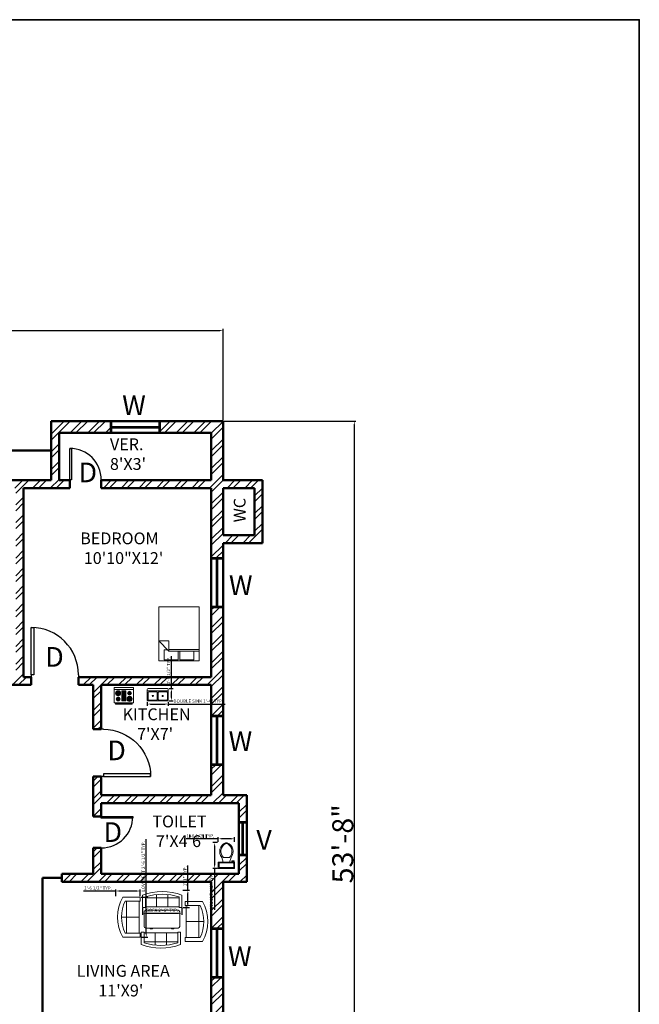
# Model space of a CAD drawing. Units: inches. Extents: x -31485 to -28799, y 18003 to 19130.
# Tile 15 of 15: x -29271 to -28799, y 18380 to 19130. Entities that reach past the tile are written whole.
import ezdxf

# ---------------------------------------------------------------- set-up
doc = ezdxf.new("R2010")
doc.units = ezdxf.units.IN
for name, color, linetype, lineweight in [('A-ANNO-DIMS', 2, 'Continuous', 18), ('A-ANNO-TEXT', 7, 'Continuous', 18), ('A-ANNO-TTLB', 7, 'Continuous', 35), ('A-AREA-IDEN', 7, 'Continuous', 18), ('A-DOOR', 3, 'Continuous', 25), ('A-FLOR-FIXT', 9, 'Continuous', 18), ('A-FURN', 8, 'Continuous', 18), ('A-GLAZ', 4, 'Continuous', 25), ('A-WALL', 7, 'Continuous', 50), ('A-WALL-PATT', 8, 'Continuous', 13)]:
    doc.layers.add(name, color=color, linetype=linetype, lineweight=lineweight)
doc.styles.get("Standard").update_dxf_attribs({"font": 'arial.ttf'})
doc.dimstyles.new('ISO-25', dxfattribs={"dimtxt": 2.5, "dimasz": 2.5, "dimexe": 1.25, "dimexo": 0.625, "dimtad": 1, "dimdec": 0, "dimlunit": 3, "dimtxsty": 'Standard', "dimcen": 2.5, "dimadec": 0, "dimazin": 0, "dimtfac": 1, "dimtdec": 0, "dimtmove": 0, "dimatfit": 3, "dimfxl": 1, "dimarcsym": 0})

# ---------------------------------------------------------------- blocks, each defined once
blk = doc.blocks.new('*U8')
for p, q in [((0, 0), (0, -100)), ((750, 0), (750, -100))]:
    blk.add_line(p, q)
blk.add_lwpolyline([(0, 0), (0, 750), (43.75, 750), (43.75, 0)], close=True)
blk.add_arc((0, 0), 750, 0, 90)
blk = doc.blocks.new('Bed - Queen')
for p, q in [((0, -80.00003), (0, 0)), ((0, 0), (59.99999, 0)), ((59.99999, 0), (59.99999, -80.00003)), ((0, -14.4), (44.8, -14.4)), ((7.99999, -1.2), (28.79998, -1.2)), ((7.99999, -14.4), (7.99999, -1.2)), ((28.79998, -1.2), (28.79998, -14.4)), ((31.19999, -1.2), (51.99999, -1.2)), ((31.19999, -14.4), (31.19999, -1.2)), ((59.99999, -29.6), (44.8, -14.4)), ((44.8, -14.4), (44.8, -29.6)), ((51.99999, -1.2), (51.99999, -16.4)), ((44.8, -16.8), (0, -16.8)), ((51.99999, -16.4), (46.79936, -16.4)), ((44.8, -29.6), (59.99999, -29.6)), ((59.99999, -80.00003), (0, -80.00003))]:
    blk.add_line(p, q)
blk = doc.blocks.new('Range-Oven - 30 in top')
for p, q in [((0, -3), (30, -3)), ((12, -6), (18, -6)), ((13, -20), (13, -6)), ((14, -6), (14, -20)), ((15, -20), (15, -6)), ((16, -6), (16, -20)), ((17, -20), (17, -6)), ((6, -24), (6, -25)), ((8, -25), (8, -24)), ((18, -20), (12, -20)), ((22, -25), (22, -24)), ((24, -24), (24, -25))]:
    blk.add_line(p, q)
for points in [[(0, -24), (0, 0), (30, 0), (30, -24)], [(12, -21), (12, -5), (18, -5), (18, -21)], [(2, -26), (2, -25), (28, -25), (28, -26)]]:
    blk.add_lwpolyline(points, close=True)
for centre, radius in [((6, -9), 4), ((6, -9), 3), ((6, -18), 3), ((6, -9), 2), ((6, -9), 1), ((24, -18), 4), ((24, -9), 3), ((24, -18), 3), ((24, -9), 2), ((24, -9), 1), ((6, -18), 2), ((6, -18), 1), ((24, -18), 2), ((24, -18), 1)]:
    blk.add_circle(centre, radius)
blk = doc.blocks.new('Sink-double - 36 in top')
for p, q in [((-18, -4), (18, -4)), ((-0.75, -18.5), (-0.75, -6.5)), ((0.75, -6.5), (0.75, -18.5))]:
    blk.add_line(p, q)
for points in [[(-16.5, 0), (16.5, 0)], [(-18, -19.5), (-18, -1.5)], [(-16.5, -18.5), (-16.5, -6.5)], [(-15.5, -5.5), (-1.75, -5.5)], [(1.75, -5.5), (15.5, -5.5)], [(16.5, -6.5), (16.5, -18.5)], [(18, -1.5), (18, -19.5)], [(16.5, -21), (-16.5, -21)], [(-1.75, -19.5), (-15.5, -19.5)], [(15.5, -19.5), (1.75, -19.5)]]:
    blk.add_lwpolyline(points)
for centre, radius in [((-8.5, -12.5), 1), ((-8.5, -12.5), 0.5), ((8.5, -12.5), 1), ((8.5, -12.5), 0.5)]:
    blk.add_circle(centre, radius)
for centre, radius, start, end in [((-16.5, -1.5), 1.5, 90, 180), ((16.5, -1.5), 1.5, 0, 90), ((-15.5, -6.5), 1, 90, 180), ((-1.75, -6.5), 1, 0, 90), ((1.75, -6.5), 1, 90, 180), ((15.5, -6.5), 1, 0, 90), ((-16.5, -19.5), 1.5, 180, 270), ((-15.5, -18.5), 1, 180, 270), ((-1.75, -18.5), 1, 270, 0), ((1.75, -18.5), 1, 180, 270), ((15.5, -18.5), 1, 270, 0), ((16.5, -19.5), 1.5, 270, 0)]:
    blk.add_arc(centre, radius, start, end)
blk = doc.blocks.new('Toilet - top')
for p, q in [((-10, -8.5), (-8, -8.5)), ((-10, -9.5), (-10, -8.5)), ((-7, -9.5), (-10, -9.5)), ((-8, -8.5), (-8, -8)), ((-7, -8), (-7, -9.5)), ((-4, -8), (-6, -14)), ((4, -8), (6, -14)), ((9.5, -6), (9.5, -2)), ((4, -14), (-4, -14))]:
    blk.add_line(p, q)
blk.add_lwpolyline([(10.5, -8), (10.5, 0), (-10.5, 0), (-10.5, -8)], close=True)
for points in [[(-9.5, -2), (-9.5, -6)], [(8.5, -1), (-8.5, -1)], [(-8.5, -7), (8.5, -7)]]:
    blk.add_lwpolyline(points)
for centre, radius, start, end in [((-8.6, -1.9), 0.884, 81.8699, 188.1301), ((-8.6, -6.1), 0.884, 171.8699, 278.1301), ((8.6, -1.9), 0.884, 351.8699, 98.1301), ((8.6, -6.1), 0.884, 261.8699, 8.1301), ((3.5, -21.6), 12.2, 141.4691, 247.9714), ((4.2, -21.8), 11.3, 136.3677, 238.9468), ((-3.5, -21.6), 12.2, 292.0284, 38.5307), ((-4.2, -21.8), 11.3, 301.053, 43.6321), ((0, -27.9), 4, 245.7318, 294.2682), ((0, -29), 4, 254.8605, 285.1395)]:
    blk.add_arc(centre, radius, start, end)
blk = doc.blocks.new('Desk - 30 x 60 in.')
for p, q in [((-26.999995, 0), (26.999995, 0)), ((-29.999995, -27), (-29.999995, -3)), ((29.999995, -3), (29.999995, -27)), ((26.999995, -30), (-26.999995, -30)), ((-20.000005, -30), (-20.000005, -31)), ((-20.000005, -31), (-16.000005, -31)), ((-16.000005, -31), (-16.000005, -30)), ((15.999995, -31), (15.999995, -30)), ((19.999995, -31), (15.999995, -31)), ((19.999995, -30), (19.999995, -31))]:
    blk.add_line(p, q)
for centre, start, end in [((-26.499995, -3.5), 98.1301, 171.8699), ((26.499995, -3.5), 8.130102, 81.8699), ((-26.499995, -26.5), 188.1301, 261.8699), ((26.499995, -26.5), 278.1301, 351.8699)]:
    blk.add_arc(centre, 3.535534, start, end)
blk = doc.blocks.new('Sofa - Roundback 7 ft.')
for p, q in [((-36.000027, -34), (-36.000027, -11.4696)), ((-35.999844, -13.3819), (35.9998, -13.3819)), ((-12.00002, -32.4421), (-12.00003, -6.5971)), ((11.99997, -32.4421), (11.99998, -6.5971)), ((35.99998, -34), (35.99998, -11.4696)), ((-36.000027, -32.4421), (35.99998, -32.4421))]:
    blk.add_line(p, q)
for points in [[(-36.000027, -34), (-42.000027, -34), (-42.000027, -8)], [(41.99998, -8), (41.99998, -34), (35.99998, -34)]]:
    blk.add_lwpolyline(points)
for centre, radius, start, end in [((0, -114.25), 114.25, 68.43141, 111.5686), ((-0.00001, -127.1968), 121.1968, 72.72033, 107.2797)]:
    blk.add_arc(centre, radius, start, end)
blk = doc.blocks.new('Sofa - Roundback Loveseat 5 ft.')
for p, q in [((-24, -33.99998), (-24, -11.46958)), ((-23.9998, -13.38178), (23.99986, -13.38178)), ((0, -32.44198), (0, -5.99998)), ((24.00004, -33.99998), (24.00004, -11.46958)), ((-24, -32.44198), (24.00004, -32.44198))]:
    blk.add_line(p, q)
for points in [[(-24, -33.99998), (-30, -33.99998), (-30, -7.99998)], [(30.00004, -7.99998), (30.00004, -33.99998), (24.00004, -33.99998)]]:
    blk.add_lwpolyline(points)
for centre, radius, start, end in [((0, -60.24998), 60.24998, 60.13715, 119.8628), ((0, -61.38438), 55.38444, 64.32083, 115.6792)]:
    blk.add_arc(centre, radius, start, end)
blk = doc.blocks.new('*D204')
at = {"layer": 'A-ANNO-DIMS', "color": 0, "lineweight": -2, "transparency": 16777216}
for p, q in [((-29663.82, 18824.74), (-29663.82, 18894.35)), ((-29661.32, 18893.1), (-29118.32, 18893.1)), ((-29115.82, 18824.74), (-29115.82, 18894.35))]:
    blk.add_line(p, q, dxfattribs=at)
at = {"layer": 'A-ANNO-DIMS', "color": 0, "transparency": 16777216}
for points in [[(-29661.32, 18893.52), (-29661.32, 18892.68), (-29663.82, 18893.1)], [(-29118.32, 18893.52), (-29118.32, 18892.68), (-29115.82, 18893.1)]]:
    blk.add_solid(points, dxfattribs=at)
at = {"layer": 'Defpoints', "color": 0, "transparency": 16777216}
for p in [(-29115.82, 18893.1), (-29663.82, 18824.12), (-29115.82, 18824.12)]:
    blk.add_point(p, dxfattribs=at)
at = {"layer": 'A-ANNO-DIMS', "color": 0, "transparency": 16777216, "insert": (-29389.82, 18901.9), "char_height": 2.5, "attachment_point": 5}
blk.add_mtext('{\\H6.4x;45\'-8"}', dxfattribs=at)
blk = doc.blocks.new('*D205')
at = {"layer": 'A-ANNO-DIMS', "color": 0, "lineweight": -2, "transparency": 16777216}
for p, q in [((-29115.2, 18824.12), (-29014.56, 18824.12)), ((-29015.81, 18821.62), (-29015.81, 18182.62)), ((-29115.2, 18180.12), (-29014.56, 18180.12))]:
    blk.add_line(p, q, dxfattribs=at)
at = {"layer": 'A-ANNO-DIMS', "color": 0, "transparency": 16777216}
for points in [[(-29016.23, 18821.62), (-29015.4, 18821.62), (-29015.81, 18824.12)], [(-29016.23, 18182.62), (-29015.4, 18182.62), (-29015.81, 18180.12)]]:
    blk.add_solid(points, dxfattribs=at)
at = {"layer": 'Defpoints', "color": 0, "transparency": 16777216}
for p in [(-29115.82, 18824.12), (-29115.82, 18180.12), (-29015.81, 18180.12)]:
    blk.add_point(p, dxfattribs=at)
at = {"layer": 'A-ANNO-DIMS', "color": 0, "transparency": 16777216, "insert": (-29024.61, 18502.12), "char_height": 2.5, "attachment_point": 5, "rotation": 90}
blk.add_mtext('{\\H6.4x;53\'-8"}', dxfattribs=at)
blk = doc.blocks.new('WIN-900-W9')
for p, q in [((-29982.21, 18824.12), (-29982.21, 18815.12)), ((-29981.21, 18824.12), (-29981.21, 18815.12)), ((-29981.21, 18820.12), (-29945.21, 18820.12)), ((-29945.21, 18824.12), (-29945.21, 18815.12)), ((-29944.21, 18824.12), (-29944.21, 18815.12)), ((-29981.21, 18819.62), (-29945.21, 18819.62)), ((-29981.21, 18819.12), (-29945.21, 18819.12))]:
    blk.add_line(p, q)
blk = doc.blocks.new('VENT-600-W6')
for p, q in [((-29884.21, 18519.12), (-29878.21, 18519.12)), ((-29884.21, 18518.12), (-29878.21, 18518.12)), ((-29881.71, 18494.12), (-29881.71, 18518.12)), ((-29881.21, 18494.12), (-29881.21, 18518.12)), ((-29880.71, 18494.12), (-29880.71, 18518.12)), ((-29884.21, 18494.12), (-29878.21, 18494.12)), ((-29884.21, 18493.12), (-29878.21, 18493.12))]:
    blk.add_line(p, q)
blk = doc.blocks.new('*D228')
at = {"layer": 'A-ANNO-DIMS', "color": 0, "lineweight": -2, "transparency": 16777216}
for p, q in [((-29174.38, 18461.57), (-29174.38, 18505.68)), ((-29178.34, 18461.57), (-29173.13, 18461.57)), ((-29174.38, 18433.51), (-29174.38, 18459.07)), ((-29178.34, 18431.01), (-29173.13, 18431.01))]:
    blk.add_line(p, q, dxfattribs=at)
at = {"layer": 'A-ANNO-DIMS', "color": 0, "transparency": 16777216}
for points in [[(-29174.8, 18459.07), (-29173.96, 18459.07), (-29174.38, 18461.57)], [(-29174.8, 18433.51), (-29173.96, 18433.51), (-29174.38, 18431.01)]]:
    blk.add_solid(points, dxfattribs=at)
at = {"layer": 'Defpoints', "color": 0, "transparency": 16777216}
for p in [(-29178.96, 18461.57), (-29174.38, 18461.57), (-29178.96, 18431.01)]:
    blk.add_point(p, dxfattribs=at)
at = {"layer": 'A-ANNO-DIMS', "color": 0, "transparency": 16777216, "insert": (-29176.3, 18484.88), "char_height": 2.5, "attachment_point": 5, "rotation": 90}
blk.add_mtext('LOVESEAT 2\'-6 1/2" TYP.', dxfattribs=at)
blk = doc.blocks.new('*D229')
at = {"layer": 'A-ANNO-DIMS', "color": 0, "lineweight": -2, "transparency": 16777216}
for p, q in [((-29197.64, 18462.2), (-29197.64, 18467.41)), ((-29178.96, 18462.2), (-29178.96, 18467.41)), ((-29197.64, 18466.16), (-29222.22, 18466.16)), ((-29181.46, 18466.16), (-29195.14, 18466.16))]:
    blk.add_line(p, q, dxfattribs=at)
at = {"layer": 'A-ANNO-DIMS', "color": 0, "transparency": 16777216}
for points in [[(-29195.14, 18466.57), (-29195.14, 18465.74), (-29197.64, 18466.16)], [(-29181.46, 18466.57), (-29181.46, 18465.74), (-29178.96, 18466.16)]]:
    blk.add_solid(points, dxfattribs=at)
at = {"layer": 'Defpoints', "color": 0, "transparency": 16777216}
for p in [(-29197.64, 18466.16), (-29197.64, 18461.57), (-29178.96, 18461.57)]:
    blk.add_point(p, dxfattribs=at)
at = {"layer": 'A-ANNO-DIMS', "color": 0, "transparency": 16777216, "insert": (-29211.18, 18468.07), "char_height": 2.5, "attachment_point": 5}
blk.add_mtext('1\'-6 1/2" TYP.', dxfattribs=at)
blk = doc.blocks.new('*D234')
at = {"layer": 'A-ANNO-DIMS', "color": 0, "lineweight": -2, "transparency": 16777216}
for p, q in [((-29177.16, 18453.04), (-29177.16, 18447.92)), ((-29147.18, 18453.04), (-29147.18, 18447.92)), ((-29174.66, 18449.17), (-29149.68, 18449.17))]:
    blk.add_line(p, q, dxfattribs=at)
at = {"layer": 'A-ANNO-DIMS', "color": 0, "transparency": 16777216}
for points in [[(-29174.66, 18449.59), (-29174.66, 18448.75), (-29177.16, 18449.17)], [(-29149.68, 18449.59), (-29149.68, 18448.75), (-29147.18, 18449.17)]]:
    blk.add_solid(points, dxfattribs=at)
at = {"layer": 'Defpoints', "color": 0, "transparency": 16777216}
for p in [(-29177.16, 18453.67), (-29147.18, 18453.67), (-29147.18, 18449.17)]:
    blk.add_point(p, dxfattribs=at)
at = {"layer": 'A-ANNO-DIMS', "color": 0, "transparency": 16777216, "insert": (-29162.17, 18451.09), "char_height": 2.5, "attachment_point": 5}
blk.add_mtext('SOFA 2\'-6" TYP.', dxfattribs=at)
blk = doc.blocks.new('*D235')
at = {"layer": 'A-ANNO-DIMS', "color": 0, "lineweight": -2, "transparency": 16777216}
for p, q in [((-29142.68, 18466.76), (-29142.68, 18485.51)), ((-29146.55, 18466.76), (-29141.43, 18466.76)), ((-29142.68, 18456.17), (-29142.68, 18464.26)), ((-29146.55, 18453.67), (-29141.43, 18453.67))]:
    blk.add_line(p, q, dxfattribs=at)
at = {"layer": 'A-ANNO-DIMS', "color": 0, "transparency": 16777216}
for points in [[(-29143.1, 18464.26), (-29142.26, 18464.26), (-29142.68, 18466.76)], [(-29143.1, 18456.17), (-29142.26, 18456.17), (-29142.68, 18453.67)]]:
    blk.add_solid(points, dxfattribs=at)
at = {"layer": 'Defpoints', "color": 0, "transparency": 16777216}
for p in [(-29147.18, 18466.76), (-29142.68, 18466.76), (-29147.18, 18453.67)]:
    blk.add_point(p, dxfattribs=at)
at = {"layer": 'A-ANNO-DIMS', "color": 0, "transparency": 16777216, "insert": (-29144.56, 18477.38), "char_height": 2.5, "attachment_point": 5, "rotation": 90}
blk.add_mtext('1\'-1" TYP.', dxfattribs=at)
blk = doc.blocks.new('*D238')
at = {"layer": 'A-ANNO-DIMS', "color": 0, "lineweight": -2, "transparency": 16777216}
for p, q in [((-29120.12, 18503), (-29123.68, 18503)), ((-29122.43, 18500.5), (-29122.43, 18485.92)), ((-29120.12, 18483.42), (-29123.68, 18483.42)), ((-29122.43, 18483.42), (-29122.43, 18451.71))]:
    blk.add_line(p, q, dxfattribs=at)
at = {"layer": 'A-ANNO-DIMS', "color": 0, "transparency": 16777216}
for points in [[(-29122.85, 18500.5), (-29122.02, 18500.5), (-29122.43, 18503)], [(-29122.85, 18485.92), (-29122.02, 18485.92), (-29122.43, 18483.42)]]:
    blk.add_solid(points, dxfattribs=at)
at = {"layer": 'Defpoints', "color": 0, "transparency": 16777216}
for p in [(-29119.5, 18503), (-29122.43, 18483.42), (-29119.5, 18483.42)]:
    blk.add_point(p, dxfattribs=at)
at = {"layer": 'A-ANNO-DIMS', "color": 0, "transparency": 16777216, "insert": (-29124.35, 18466.31), "char_height": 2.5, "attachment_point": 5, "rotation": 90}
blk.add_mtext('WC 1\'-7 1/2" TYP.', dxfattribs=at)
blk = doc.blocks.new('*D239')
at = {"layer": 'A-ANNO-DIMS', "color": 0, "lineweight": -2, "transparency": 16777216}
for p, q in [((-29119.5, 18505.94), (-29144.08, 18505.94)), ((-29119.5, 18503.63), (-29119.5, 18507.19)), ((-29109.55, 18505.94), (-29117, 18505.94)), ((-29107.05, 18503.63), (-29107.05, 18507.19))]:
    blk.add_line(p, q, dxfattribs=at)
at = {"layer": 'A-ANNO-DIMS', "color": 0, "transparency": 16777216}
for points in [[(-29117, 18506.35), (-29117, 18505.52), (-29119.5, 18505.94)], [(-29109.55, 18506.35), (-29109.55, 18505.52), (-29107.05, 18505.94)]]:
    blk.add_solid(points, dxfattribs=at)
at = {"layer": 'Defpoints', "color": 0, "transparency": 16777216}
for p in [(-29119.5, 18505.94), (-29119.5, 18503), (-29107.05, 18503)]:
    blk.add_point(p, dxfattribs=at)
at = {"layer": 'A-ANNO-DIMS', "color": 0, "transparency": 16777216, "insert": (-29133.04, 18507.86), "char_height": 2.5, "attachment_point": 5}
blk.add_mtext('1\'-0 1/2" TYP.', dxfattribs=at)
blk = doc.blocks.new('*D256')
at = {"layer": 'A-ANNO-DIMS', "color": 0, "lineweight": -2, "transparency": 16777216}
for p, q in [((-29173.6, 18610.35), (-29173.6, 18607.32)), ((-29157.59, 18610.35), (-29157.59, 18607.32)), ((-29171.1, 18608.57), (-29160.09, 18608.57)), ((-29157.59, 18608.57), (-29114.28, 18608.57))]:
    blk.add_line(p, q, dxfattribs=at)
at = {"layer": 'A-ANNO-DIMS', "color": 0, "transparency": 16777216}
for points in [[(-29171.1, 18608.99), (-29171.1, 18608.16), (-29173.6, 18608.57)], [(-29160.09, 18608.99), (-29160.09, 18608.16), (-29157.59, 18608.57)]]:
    blk.add_solid(points, dxfattribs=at)
at = {"layer": 'Defpoints', "color": 0, "transparency": 16777216}
for p in [(-29173.6, 18610.98), (-29157.59, 18610.98), (-29157.59, 18608.57)]:
    blk.add_point(p, dxfattribs=at)
at = {"layer": 'A-ANNO-DIMS', "color": 0, "transparency": 16777216, "insert": (-29134.69, 18610.49), "char_height": 2.5, "attachment_point": 5}
blk.add_mtext('DOUBLE SINK 1\'-4" TYP.', dxfattribs=at)
blk = doc.blocks.new('*D257')
at = {"layer": 'A-ANNO-DIMS', "color": 0, "lineweight": -2, "transparency": 16777216}
for p, q in [((-29155.19, 18620.31), (-29155.19, 18645.13)), ((-29156.97, 18620.31), (-29153.94, 18620.31)), ((-29155.19, 18613.48), (-29155.19, 18617.81)), ((-29156.97, 18610.98), (-29153.94, 18610.98))]:
    blk.add_line(p, q, dxfattribs=at)
at = {"layer": 'A-ANNO-DIMS', "color": 0, "transparency": 16777216}
for points in [[(-29155.61, 18617.81), (-29154.78, 18617.81), (-29155.19, 18620.31)], [(-29155.61, 18613.48), (-29154.78, 18613.48), (-29155.19, 18610.98)]]:
    blk.add_solid(points, dxfattribs=at)
at = {"layer": 'Defpoints', "color": 0, "transparency": 16777216}
for p in [(-29157.59, 18620.31), (-29155.19, 18620.31), (-29157.59, 18610.98)]:
    blk.add_point(p, dxfattribs=at)
at = {"layer": 'A-ANNO-DIMS', "color": 0, "transparency": 16777216, "insert": (-29157.11, 18633.97), "char_height": 2.5, "attachment_point": 5, "rotation": 90}
blk.add_mtext('0\'-9 1/2" TYP.', dxfattribs=at)

msp = doc.modelspace()

# ---------------------------------------------------------------- hatches: boundary and pattern name
at = {"layer": 'A-WALL-PATT'}
h = msp.add_hatch(dxfattribs=at)
h.set_pattern_fill('ANSI32', color=256)
h.set_pattern_definition([(45, (-227.67, 0), (-6.735192, 6.735192), []), (45, (-223.18, 0), (-6.735192, 6.735192), [])])
h.paths.add_polyline_path([(-29507.82, 18213.12), (-29493.82, 18213.12), (-29493.82, 18219.12), (-29507.82, 18219.12), (-29507.82, 18309.12), (-29504.3, 18309.12), (-29504.3, 18315.12), (-29513.82, 18315.12), (-29513.82, 18243.12), (-29654.82, 18243.12), (-29654.82, 18265.36), (-29663.82, 18265.36), (-29663.82, 18180.12), (-29603.32, 18180.12), (-29603.32, 18189.12), (-29654.82, 18189.12), (-29654.82, 18237.12), (-29513.82, 18237.12), (-29513.82, 18189.12), (-29565.32, 18189.12), (-29565.32, 18180.12), (-29507.82, 18180.12)])
h.paths.add_polyline_path([(-29408.82, 18189.12), (-29447.82, 18189.12), (-29447.82, 18371.74), (-29453.82, 18371.74), (-29453.82, 18365.12), (-29476.66, 18365.12), (-29476.66, 18359.12), (-29453.82, 18359.12), (-29453.82, 18315.12), (-29480.3, 18315.12), (-29480.3, 18309.12), (-29453.82, 18309.12), (-29453.82, 18219.12), (-29467.82, 18219.12), (-29467.82, 18213.12), (-29453.82, 18213.12), (-29453.82, 18180.12), (-29408.82, 18180.12)])
h.paths.add_polyline_path([(-29325.82, 18213.12), (-29311.82, 18213.12), (-29311.82, 18219.12), (-29325.82, 18219.12), (-29325.82, 18309.12), (-29298.35, 18309.12), (-29298.35, 18315.12), (-29325.82, 18315.12), (-29325.82, 18359.12), (-29304.41, 18359.12), (-29304.41, 18365.12), (-29325.82, 18365.12), (-29325.82, 18371.25), (-29331.82, 18371.25), (-29331.82, 18189.12), (-29370.82, 18189.12), (-29370.82, 18180.12), (-29325.82, 18180.12)])
h.paths.add_polyline_path([(-29265.82, 18237.12), (-29124.82, 18237.12), (-29124.82, 18189.12), (-29176.32, 18189.12), (-29176.32, 18180.12), (-29115.82, 18180.12), (-29115.82, 18268.84), (-29124.82, 18268.84), (-29124.82, 18243.12), (-29265.82, 18243.12), (-29265.82, 18315.12), (-29274.35, 18315.12), (-29274.35, 18309.12), (-29271.82, 18309.12), (-29271.82, 18219.12), (-29285.82, 18219.12), (-29285.82, 18213.12), (-29271.82, 18213.12), (-29271.82, 18180.12), (-29214.32, 18180.12), (-29214.32, 18189.12), (-29265.82, 18189.12)])
h.paths.add_polyline_path([(-29209.82, 18365.12), (-29262.82, 18365.12), (-29268.41, 18365.12), (-29268.41, 18359.12), (-29209.82, 18359.12)])
h.paths.add_polyline_path([(-29085.82, 18365.12), (-29115.82, 18365.12), (-29115.82, 18400.12), (-29124.82, 18400.12), (-29124.82, 18365.12), (-29171.82, 18365.12), (-29171.82, 18359.12), (-29124.82, 18359.12), (-29124.82, 18306.84), (-29115.82, 18306.84), (-29115.82, 18317.12), (-29085.82, 18317.12)])
h.paths.add_polyline_path([(-29115.82, 18359.12), (-29091.82, 18359.12), (-29091.82, 18323.12), (-29115.82, 18323.12)], flags=16)
h.paths.add_polyline_path([(-29607.82, 18365.12), (-29654.82, 18365.12), (-29654.82, 18400.12), (-29663.82, 18400.12), (-29663.82, 18365.12), (-29693.82, 18365.12), (-29693.82, 18317.12), (-29663.82, 18317.12), (-29663.82, 18303.36), (-29654.82, 18303.36), (-29654.82, 18359.12), (-29607.82, 18359.12)])
h.paths.add_polyline_path([(-29663.82, 18359.12), (-29663.82, 18323.12), (-29687.82, 18323.12), (-29687.82, 18359.12)], flags=16)
h.paths.add_polyline_path([(-29512.66, 18365.12), (-29516.82, 18365.12), (-29569.82, 18365.12), (-29569.82, 18359.12), (-29512.66, 18359.12)])
h.paths.add_polyline_path([(-29654.82, 18473.12), (-29553.73, 18473.12), (-29553.73, 18479.12), (-29564.82, 18479.12), (-29564.82, 18500.25), (-29569.57, 18500.25, -0.011537), (-29570.67, 18500.25), (-29570.82, 18500.25), (-29570.82, 18479.12), (-29675.82, 18479.12), (-29675.82, 18493.12), (-29681.82, 18493.12), (-29681.82, 18473.12), (-29663.82, 18473.12), (-29663.82, 18438.12), (-29654.82, 18438.12)])
h.paths.add_polyline_path([(-29564.82, 18547.44), (-29570.82, 18547.44), (-29570.82, 18539.12), (-29654.82, 18539.12), (-29654.82, 18562.12), (-29663.82, 18562.12), (-29663.82, 18539.12), (-29681.82, 18539.12), (-29681.82, 18519.12), (-29675.82, 18519.12), (-29675.82, 18533.12), (-29570.82, 18533.12), (-29570.82, 18524.25), (-29564.82, 18524.25)])
h.paths.add_polyline_path([(-29563.19, 18629.12), (-29654.82, 18629.12), (-29654.82, 18682.12), (-29663.82, 18682.12), (-29663.82, 18600.12), (-29654.82, 18600.12), (-29654.82, 18623.12), (-29570.82, 18623.12), (-29570.82, 18583.44), (-29566.85, 18583.44), (-29564.82, 18583.44), (-29564.82, 18623.12), (-29563.19, 18623.12)])
h.paths.add_polyline_path([(-29315.33, 18629.12), (-29396.82, 18629.12), (-29396.82, 18682.12), (-29402.82, 18682.12), (-29402.82, 18629.12), (-29482.28, 18629.12), (-29482.28, 18626.12), (-29482.28, 18623.12), (-29402.82, 18623.12), (-29402.82, 18416.12), (-29453.82, 18416.12), (-29453.82, 18407.74), (-29447.82, 18407.74), (-29447.82, 18410.12), (-29331.82, 18410.12), (-29331.82, 18407.25), (-29325.82, 18407.25), (-29325.82, 18416.12), (-29396.82, 18416.12), (-29396.82, 18623.12), (-29315.33, 18623.12)])
h.paths.add_polyline_path([(-29525.82, 18773.12), (-29492.32, 18773.12), (-29492.32, 18779.12), (-29498.82, 18779.12), (-29498.82, 18815.12), (-29469.82, 18815.12), (-29469.82, 18824.12), (-29504.82, 18824.12), (-29504.82, 18779.12), (-29552.82, 18779.12), (-29552.82, 18824.12), (-29587.82, 18824.12), (-29587.82, 18815.12), (-29558.82, 18815.12), (-29558.82, 18779.12), (-29563.08, 18779.12), (-29563.08, 18776.12), (-29563.08, 18773.12), (-29531.82, 18773.12), (-29531.82, 18629.12), (-29533.3, 18629.12), (-29533.3, 18626.12), (-29533.3, 18623.12), (-29518.28, 18623.12), (-29518.28, 18629.12), (-29525.82, 18629.12)])
h.paths.add_polyline_path([(-29654.82, 18779.12), (-29654.82, 18815.12), (-29625.82, 18815.12), (-29625.82, 18824.12), (-29663.82, 18824.12), (-29663.82, 18779.12), (-29693.82, 18779.12), (-29693.82, 18731.12), (-29663.82, 18731.12), (-29663.82, 18720.12), (-29654.82, 18720.12), (-29654.82, 18773.12), (-29587.08, 18773.12), (-29587.08, 18779.12)])
h.paths.add_polyline_path([(-29663.82, 18773.12), (-29663.82, 18737.12), (-29687.82, 18737.12), (-29687.82, 18773.12)], flags=16)
h.paths.add_polyline_path([(-29396.82, 18815.12), (-29367.82, 18815.12), (-29367.82, 18824.12), (-29431.82, 18824.12), (-29431.82, 18815.12), (-29402.82, 18815.12), (-29402.82, 18779.12), (-29468.32, 18779.12), (-29468.32, 18776.12), (-29468.32, 18773.12), (-29402.82, 18773.12), (-29402.82, 18720.12), (-29396.82, 18720.12), (-29396.82, 18773.12), (-29331.17, 18773.12), (-29331.17, 18779.12), (-29396.82, 18779.12)])
h.paths.add_polyline_path([(-29232.68, 18779.12), (-29240.82, 18779.12), (-29240.82, 18815.12), (-29201.82, 18815.12), (-29201.82, 18824.12), (-29246.82, 18824.12), (-29246.82, 18779.12), (-29294.82, 18779.12), (-29294.82, 18824.12), (-29329.82, 18824.12), (-29329.82, 18815.12), (-29300.82, 18815.12), (-29300.82, 18779.12), (-29307.17, 18779.12), (-29307.17, 18776.12), (-29307.17, 18773.12), (-29273.82, 18773.12), (-29273.82, 18629.12), (-29279.33, 18629.12), (-29279.33, 18626.12), (-29279.33, 18623.12), (-29262.04, 18623.12), (-29262.04, 18629.12), (-29267.82, 18629.12), (-29267.82, 18773.12), (-29232.68, 18773.12)])
h.paths.add_polyline_path([(-29085.82, 18779.12), (-29115.82, 18779.12), (-29115.82, 18824.12), (-29163.82, 18824.12), (-29163.82, 18815.12), (-29124.82, 18815.12), (-29124.82, 18779.12), (-29208.68, 18779.12), (-29208.68, 18776.12), (-29208.68, 18773.12), (-29124.82, 18773.12), (-29124.82, 18720.12), (-29115.82, 18720.12), (-29115.82, 18731.12), (-29085.82, 18731.12)])
h.paths.add_polyline_path([(-29115.82, 18773.12), (-29091.82, 18773.12), (-29091.82, 18737.12), (-29115.82, 18737.12)], flags=16)
h.paths.add_polyline_path([(-29115.82, 18682.12), (-29124.82, 18682.12), (-29124.82, 18629.12), (-29226.04, 18629.12), (-29226.04, 18626.12), (-29226.04, 18623.12), (-29214.82, 18623.12), (-29214.82, 18589.35), (-29208.82, 18589.35), (-29208.82, 18623.12), (-29124.82, 18623.12), (-29124.82, 18600.12), (-29115.82, 18600.12)])
h.paths.add_polyline_path([(-29115.82, 18562.12), (-29124.82, 18562.12), (-29124.82, 18539.12), (-29208.82, 18539.12), (-29208.82, 18553.35), (-29211.82, 18553.35), (-29214.82, 18553.35), (-29214.82, 18522.99), (-29208.82, 18522.99), (-29208.82, 18533.12), (-29103.82, 18533.12), (-29103.82, 18519.12), (-29097.82, 18519.12), (-29097.82, 18539.12), (-29115.82, 18539.12)])
h.paths.add_polyline_path([(-29115.82, 18473.12), (-29097.82, 18473.12), (-29097.82, 18493.12), (-29103.82, 18493.12), (-29103.82, 18479.12), (-29208.82, 18479.12), (-29208.82, 18498.99), (-29214.82, 18498.99), (-29214.82, 18479.12), (-29238.82, 18479.12), (-29238.82, 18473.12), (-29124.82, 18473.12), (-29124.82, 18438.12), (-29115.82, 18438.12)])
h.paths.add_polyline_path([(-29513.85, 18245.24), (-29448.79, 18245.24), (-29448.79, 18278.82), (-29513.85, 18278.82)], flags=9)
h.paths.add_polyline_path([(-29331.85, 18241.25), (-29266.79, 18241.25), (-29266.79, 18274.84), (-29331.85, 18274.84)], flags=9)
h.paths.add_polyline_path([(-29095.1, 18330.99), (-29095.1, 18356.44), (-29113.65, 18356.44), (-29113.65, 18330.99)], flags=8)
h.paths.add_polyline_path([(-29666.32, 18333.81), (-29666.32, 18359.25), (-29684.87, 18359.25), (-29684.87, 18333.81)], flags=24)
h.paths.add_polyline_path([(-29665.76, 18745.92), (-29665.76, 18771.37), (-29684.31, 18771.37), (-29684.31, 18745.92)], flags=8)
h.paths.add_polyline_path([(-29093.62, 18744.62), (-29093.62, 18770.06), (-29112.17, 18770.06), (-29112.17, 18744.62)], flags=8)

# ---------------------------------------------------------------- linework, layer by layer
at = {"layer": 'A-ANNO-TTLB'}
msp.add_lwpolyline([(-31485.1, 19129.94), (-28798.64, 19129.94), (-28798.64, 18002.86), (-31485.1, 18002.86)], close=True, dxfattribs=at)
at = {"layer": 'A-WALL'}
for p, q in [((-29246.82, 18779.12), (-29246.82, 18824.12)), ((-29246.82, 18824.12), (-29115.82, 18824.12)), ((-29115.82, 18824.12), (-29115.82, 18779.12)), ((-29240.82, 18779.12), (-29240.82, 18815.12)), ((-29240.82, 18815.12), (-29124.82, 18815.12)), ((-29124.82, 18815.12), (-29124.82, 18779.12)), ((-29294.82, 18801.62), (-29246.82, 18801.62)), ((-29294.82, 18779.12), (-29246.82, 18779.12)), ((-29240.82, 18779.12), (-29232.68, 18779.12)), ((-29232.68, 18779.12), (-29232.68, 18773.12)), ((-29208.68, 18779.12), (-29208.68, 18773.12)), ((-29208.68, 18779.12), (-29124.82, 18779.12)), ((-29115.82, 18779.12), (-29085.82, 18779.12)), ((-29085.82, 18779.12), (-29085.82, 18731.12)), ((-29267.82, 18629.12), (-29267.82, 18773.12)), ((-29267.82, 18773.12), (-29232.68, 18773.12)), ((-29208.68, 18773.12), (-29124.82, 18773.12)), ((-29124.82, 18773.12), (-29124.82, 18629.12)), ((-29115.82, 18773.12), (-29115.82, 18737.12)), ((-29115.82, 18773.12), (-29091.82, 18773.12)), ((-29091.82, 18773.12), (-29091.82, 18737.12)), ((-29115.82, 18737.12), (-29091.82, 18737.12)), ((-29115.82, 18731.12), (-29085.82, 18731.12)), ((-29115.82, 18731.12), (-29115.82, 18539.12)), ((-29267.82, 18629.12), (-29262.04, 18629.12)), ((-29262.04, 18629.12), (-29262.04, 18623.12)), ((-29226.04, 18629.12), (-29226.04, 18623.12)), ((-29226.04, 18629.12), (-29124.82, 18629.12)), ((-29279.33, 18623.12), (-29262.04, 18623.12)), ((-29226.04, 18623.12), (-29214.82, 18623.12)), ((-29214.82, 18623.12), (-29214.82, 18589.35)), ((-29208.82, 18623.12), (-29208.82, 18589.35)), ((-29208.82, 18623.12), (-29124.82, 18623.12)), ((-29124.82, 18623.12), (-29124.82, 18539.12)), ((-29214.82, 18589.35), (-29208.82, 18589.35)), ((-29214.82, 18553.35), (-29208.82, 18553.35)), ((-29214.82, 18553.35), (-29214.82, 18522.99)), ((-29208.82, 18553.35), (-29208.82, 18539.12)), ((-29208.82, 18539.12), (-29124.82, 18539.12)), ((-29115.82, 18539.12), (-29097.82, 18539.12)), ((-29097.82, 18539.12), (-29097.82, 18473.12)), ((-29208.82, 18533.12), (-29103.82, 18533.12)), ((-29208.82, 18533.12), (-29208.82, 18522.99)), ((-29103.82, 18533.12), (-29103.82, 18479.12)), ((-29214.82, 18522.99), (-29208.82, 18522.99)), ((-29214.82, 18498.99), (-29208.82, 18498.99)), ((-29214.82, 18498.99), (-29214.82, 18479.12)), ((-29208.82, 18498.99), (-29208.82, 18479.12)), ((-29238.82, 18476.12), (-29253.51, 18476.12)), ((-29253.51, 18476.12), (-29253.51, 18365.12)), ((-29238.82, 18479.12), (-29214.82, 18479.12)), ((-29238.82, 18479.12), (-29238.82, 18473.12)), ((-29208.82, 18479.12), (-29103.82, 18479.12)), ((-29238.82, 18473.12), (-29124.82, 18473.12)), ((-29124.82, 18473.12), (-29124.82, 18365.12)), ((-29115.82, 18473.12), (-29115.82, 18365.12)), ((-29115.82, 18473.12), (-29097.82, 18473.12)), ((-29124.82, 18419.12), (-29124.82, 18419.12))]:
    msp.add_line(p, q, dxfattribs=at)

# ---------------------------------------------------------------- block references
at = {"layer": 'A-DOOR'}
for p, xscale, yscale, zscale in [((-29232.68, 18779.32), 0.0320000000000009, 0.0320000000000009, 0.0320000000000009), ((-29262.04, 18630.92), 0.0480000000000013, 0.0480000000000013, 0.0480000000000013)]:
    msp.add_blockref('*U8', p, dxfattribs=dict(at, xscale=xscale, yscale=yscale, zscale=zscale))
at = {"layer": 'A-DOOR', "rotation": 270}
for p, xscale, yscale, zscale in [((-29207.02, 18553.35), -0.0480000007307817, 0.0480000007307817, 0.0480000007307817), ((-29208.62, 18522.99), 0.0319999995506959, 0.0319999995506959, 0.0319999995506959)]:
    msp.add_blockref('*U8', p, dxfattribs=dict(at, xscale=xscale, yscale=yscale, zscale=zscale))
at = {"layer": 'A-FLOR-FIXT'}
for name, p, xscale, yscale, zscale in [('Range-Oven - 30 in top', (-29198.74, 18621.2), 0.4852446628127246, 0.4852446628127246, 0.4852446628127246), ('Sink-double - 36 in top', (-29165.6, 18620.31), 0.4446151646272686, 0.4446151646272686, 0.4446151646272686)]:
    msp.add_blockref(name, p, dxfattribs=dict(at, xscale=xscale, yscale=yscale, zscale=zscale))
at = {"layer": 'A-FLOR-FIXT', "xscale": 0.5926017901613329, "yscale": 0.5926017901613329, "zscale": 0.5926017901613329, "rotation": 180}
msp.add_blockref('Toilet - top', (-29113.27, 18483.42), dxfattribs=at)
at = {"layer": 'A-FURN'}
for name, p, xscale, yscale, zscale, rotation in [('Bed - Queen', (-29134.03, 18641.53), 0.5144931166195136, 0.5144931166195136, 0.5144931166195136, 180), ('Sofa - Roundback Loveseat 5 ft.', (-29196.28, 18446.29), 0.5093827995121489, 0.5093827995121489, 0.5093827995121489, 89.99999999999999), ('Sofa - Roundback Loveseat 5 ft.', (-29127.4, 18442.9), 0.5093827995121489, 0.5093827995121489, 0.5093827995121489, 270), ('Sofa - Roundback 7 ft.', (-29163.18, 18422.63), 0.356964146635117, 0.356964146635117, 0.356964146635117, 180)]:
    msp.add_blockref(name, p, dxfattribs=dict(at, xscale=xscale, yscale=yscale, zscale=zscale, rotation=rotation))
for name, p, xscale, yscale, zscale in [('Sofa - Roundback 7 ft.', (-29162.17, 18465.8), 0.356964146635117, 0.356964146635117, 0.356964146635117), ('Desk - 30 x 60 in.', (-29162.4, 18451.54), 0.4556329481741908, 0.4556329481741908, 0.4556329481741908)]:
    msp.add_blockref(name, p, dxfattribs=dict(at, xscale=xscale, yscale=yscale, zscale=zscale))
at = {"layer": 'A-GLAZ'}
for name in ['WIN-900-W9', 'VENT-600-W6']:
    msp.add_blockref(name, (780.38, 0), dxfattribs=at)
for p, rotation in [((-10300.7, 48664.32), 89.9999999999847), ((-10300.7, 48544.32), 89.9999999999847), ((-10300.7, 48382.32), 90.00000000000547)]:
    msp.add_blockref('WIN-900-W9', p, dxfattribs=dict(at, rotation=rotation))

# ---------------------------------------------------------------- texts
at = {"layer": 'A-ANNO-TEXT', "char_height": 15, "attachment_point": 1}
for s, insert in [('{W}', (-29192.7, 18843.69)), ('{D}', (-29225.94, 18792.53)), ('{W}', (-29111.35, 18706.56)), ('{D}', (-29251.32, 18652)), ('{W}', (-29111.59, 18587.82)), ('{D}', (-29204, 18580.8)), ('{D}', (-29206.9, 18518.54)), ('{V}', (-29090.49, 18512.66)), ('{W}', (-29112.06, 18423.97))]:
    msp.add_mtext_dynamic_manual_height_columns(s, width=1534.0875, gutter_width=12.5, heights=[0], dxfattribs=dict(at, insert=insert))
at = {"layer": 'A-AREA-IDEN', "char_height": 9, "attachment_point": 1}
for s, insert in [("{VER.\\P8'X3'}", (-29202.02, 18810.98)), ('{BEDROOM\\P 10\'10"X12\'}', (-29224.69, 18739.31)), ("{  KITCHEN\\P      7'X7'}", (-29197.88, 18605.3)), ('{    TOILET\\P     7\'X4\'6"}', (-29180.7, 18523.64)), ("{LIVING AREA\\P      11'X9'}", (-29227.39, 18409.82))]:
    msp.add_mtext_dynamic_manual_height_columns(s, width=988.498, gutter_width=12.5, heights=[0], dxfattribs=dict(at, insert=insert))
at = {"layer": 'A-AREA-IDEN', "insert": (-29107.69, 18747.02), "char_height": 9, "attachment_point": 1, "rotation": 90}
msp.add_mtext_dynamic_manual_height_columns('{WC}', width=988.498, gutter_width=12.5, heights=[0], dxfattribs=at)

# ---------------------------------------------------------------- dimensions: what is measured, and where the dimension line sits
at = {"layer": 'A-ANNO-DIMS'}
for base, p1, p2, text, override, picture, middle in [((-29115.82, 18893.1), (-29663.82, 18824.12), (-29115.82, 18824.12), '{\\H6.4x;<>}', {"dimclrd": 0, "dimclre": 0, "dimclrt": 0}, '*D204', (-29389.82, 18901.9)), ((-29157.59, 18608.57), (-29173.6, 18610.98), (-29157.59, 18610.98), 'DOUBLE SINK <> TYP.', {"dimdec": 1, "dimlfac": 1, "dimrnd": 0, "dimzin": 1, "dimdsep": 46, "dimlunit": 4, "dimfrac": 2}, '*D256', (-29134.69, 18610.49)), ((-29147.18, 18449.17), (-29177.16, 18453.67), (-29147.18, 18453.67), 'SOFA <> TYP.', {"dimdec": 1, "dimlfac": 1, "dimrnd": 0, "dimzin": 1, "dimdsep": 46, "dimlunit": 4, "dimfrac": 2}, '*D234', (-29162.17, 18451.09))]:
    dim = msp.add_linear_dim(base=base, p1=p1, p2=p2, text=text, dimstyle='ISO-25', override=override, dxfattribs=at)
    dim.commit()
    dim.dimension.update_dxf_attribs({"geometry": picture, "text_midpoint": middle})
for base, p1, p2, angle, text, override, picture, middle in [((-29015.81, 18180.12), (-29115.82, 18824.12), (-29115.82, 18180.12), 90, '{\\H6.4x;<>}', {"dimclrd": 0, "dimclre": 0, "dimclrt": 0}, '*D205', (-29024.61, 18502.12)), ((-29155.19, 18620.31), (-29157.59, 18610.98), (-29157.59, 18620.31), 90, '<> TYP.', {"dimdec": 1, "dimlfac": 1, "dimrnd": 0, "dimzin": 1, "dimdsep": 46, "dimlunit": 4, "dimfrac": 2}, '*D257', (-29157.11, 18633.97)), ((-29119.4972, 18505.9379), (-29107.0525, 18503.0005), (-29119.4972, 18503.0005), 180, '<> TYP.', {"dimdec": 1, "dimlfac": 1, "dimrnd": 0, "dimzin": 1, "dimdsep": 46, "dimlunit": 4, "dimfrac": 2}, '*D239', (-29133.0366, 18507.8556)), ((-29174.38, 18461.57), (-29178.96, 18431.01), (-29178.96, 18461.57), 90, 'LOVESEAT <> TYP.', {"dimdec": 1, "dimlfac": 1, "dimrnd": 0, "dimzin": 1, "dimdsep": 46, "dimlunit": 4, "dimfrac": 2}, '*D228', (-29176.3, 18484.88)), ((-29122.43, 18483.42), (-29119.5, 18503), (-29119.5, 18483.42), 270, 'WC <> TYP.', {"dimdec": 1, "dimlfac": 1, "dimrnd": 0, "dimzin": 1, "dimdsep": 46, "dimlunit": 4, "dimfrac": 2}, '*D238', (-29124.35, 18466.31)), ((-29142.68, 18466.76), (-29147.18, 18453.67), (-29147.18, 18466.76), 90, '<> TYP.', {"dimdec": 1, "dimlfac": 1, "dimrnd": 0, "dimzin": 1, "dimdsep": 46, "dimlunit": 4, "dimfrac": 2}, '*D235', (-29144.56, 18477.38)), ((-29197.64, 18466.16), (-29178.96, 18461.57), (-29197.64, 18461.57), 180, '<> TYP.', {"dimdec": 1, "dimlfac": 1, "dimrnd": 0, "dimzin": 1, "dimdsep": 46, "dimlunit": 4, "dimfrac": 2}, '*D229', (-29211.18, 18468.07))]:
    dim = msp.add_linear_dim(base=base, p1=p1, p2=p2, angle=angle, text=text, dimstyle='ISO-25', override=override, dxfattribs=at)
    dim.commit()
    dim.dimension.update_dxf_attribs({"geometry": picture, "text_midpoint": middle})

doc.saveas('drawing.dxf')
